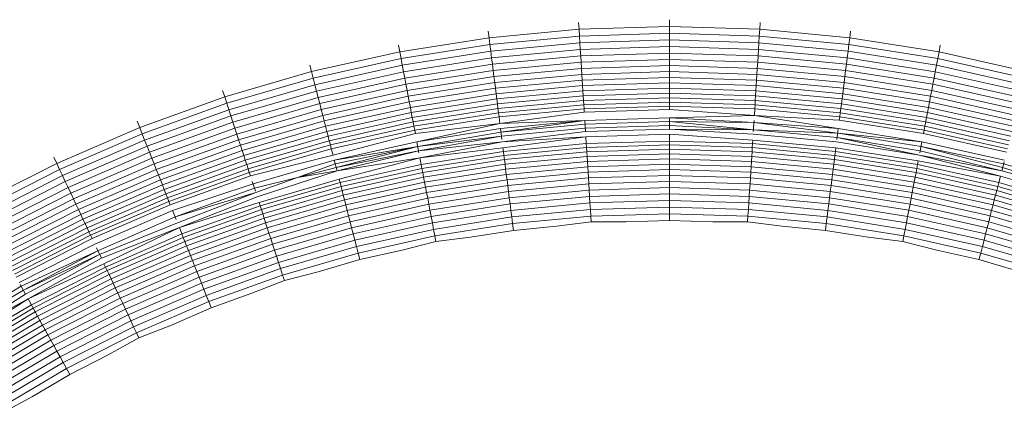
# Model space of a CAD drawing. Units: inches. Extents: x 64 to 1167, y 117 to 939.
# Tile 50 of 56: x 1130.0344 to 1130.3689, y 501.3001 to 501.4339. Entities that reach past the tile are written whole.
import ezdxf

# ---------------------------------------------------------------- set-up
doc = ezdxf.new("R2010")
doc.units = ezdxf.units.IN
doc.header["$MEASUREMENT"] = 0
doc.layers.add('A-FLOR-FIXT', color=8, linetype='Continuous', lineweight=18)

msp = doc.modelspace()

# ---------------------------------------------------------------- linework, layer by layer
at = {"layer": 'A-FLOR-FIXT'}
for p, q in [((1130.25515, 501.4316), (1130.25515, 501.43391)), ((1130.19388, 501.42774), (1130.19359, 501.43003)), ((1130.22445, 501.43064), (1130.19388, 501.42774)), ((1130.22431, 501.43294), (1130.22445, 501.43064)), ((1130.25515, 501.4316), (1130.22445, 501.43064)), ((1130.22445, 501.43064), (1130.2246, 501.42834)), ((1130.25515, 501.4293), (1130.25515, 501.4316)), ((1130.28585, 501.43064), (1130.25515, 501.4316)), ((1130.2857, 501.42834), (1130.28585, 501.43064)), ((1130.28585, 501.43064), (1130.28599, 501.43294)), ((1130.31643, 501.42774), (1130.28585, 501.43064)), ((1130.31643, 501.42774), (1130.31671, 501.43003)), ((1130.19388, 501.42774), (1130.16354, 501.42294)), ((1130.19416, 501.42546), (1130.19388, 501.42774)), ((1130.2246, 501.42834), (1130.19416, 501.42546)), ((1130.25515, 501.4293), (1130.2246, 501.42834)), ((1130.2246, 501.42834), (1130.22474, 501.42607)), ((1130.25515, 501.42702), (1130.22474, 501.42607)), ((1130.25515, 501.42702), (1130.25515, 501.4293)), ((1130.2857, 501.42834), (1130.25515, 501.4293)), ((1130.25515, 501.42477), (1130.25515, 501.42702)), ((1130.28556, 501.42607), (1130.25515, 501.42702)), ((1130.28556, 501.42607), (1130.2857, 501.42834)), ((1130.31614, 501.42546), (1130.2857, 501.42834)), ((1130.31614, 501.42546), (1130.31643, 501.42774)), ((1130.34676, 501.42294), (1130.31643, 501.42774)), ((1130.16311, 501.42521), (1130.16354, 501.42294)), ((1130.19416, 501.42546), (1130.16397, 501.42068)), ((1130.19445, 501.4232), (1130.19416, 501.42546)), ((1130.22474, 501.42607), (1130.19445, 501.4232)), ((1130.22488, 501.42382), (1130.19473, 501.42097)), ((1130.22474, 501.42607), (1130.22488, 501.42382)), ((1130.25515, 501.42477), (1130.22488, 501.42382)), ((1130.22488, 501.42382), (1130.22502, 501.42162)), ((1130.25515, 501.42256), (1130.25515, 501.42477)), ((1130.28542, 501.42382), (1130.25515, 501.42477)), ((1130.28528, 501.42162), (1130.28542, 501.42382)), ((1130.28542, 501.42382), (1130.28556, 501.42607)), ((1130.31557, 501.42097), (1130.28542, 501.42382)), ((1130.31585, 501.4232), (1130.28556, 501.42607)), ((1130.31585, 501.4232), (1130.31614, 501.42546)), ((1130.34633, 501.42068), (1130.31614, 501.42546)), ((1130.34719, 501.42521), (1130.34676, 501.42294)), ((1130.16354, 501.42294), (1130.13357, 501.41624)), ((1130.16397, 501.42068), (1130.13414, 501.41401)), ((1130.16354, 501.42294), (1130.16397, 501.42068)), ((1130.16397, 501.42068), (1130.1644, 501.41844)), ((1130.19445, 501.4232), (1130.1644, 501.41844)), ((1130.19473, 501.42097), (1130.16482, 501.41623)), ((1130.19473, 501.42097), (1130.19445, 501.4232)), ((1130.19501, 501.41878), (1130.19473, 501.42097)), ((1130.22502, 501.42162), (1130.19501, 501.41878)), ((1130.25515, 501.42256), (1130.22502, 501.42162)), ((1130.22502, 501.42162), (1130.22516, 501.41946)), ((1130.25515, 501.4204), (1130.22516, 501.41946)), ((1130.25515, 501.4204), (1130.25515, 501.42256)), ((1130.28528, 501.42162), (1130.25515, 501.42256)), ((1130.25515, 501.4183), (1130.25515, 501.4204)), ((1130.28515, 501.41946), (1130.25515, 501.4204)), ((1130.28515, 501.41946), (1130.28528, 501.42162)), ((1130.31529, 501.41878), (1130.28528, 501.42162)), ((1130.31529, 501.41878), (1130.31557, 501.42097)), ((1130.31557, 501.42097), (1130.31585, 501.4232)), ((1130.34548, 501.41623), (1130.31557, 501.42097)), ((1130.3459, 501.41844), (1130.31585, 501.4232)), ((1130.34633, 501.42068), (1130.3459, 501.41844)), ((1130.34676, 501.42294), (1130.34633, 501.42068)), ((1130.37616, 501.41401), (1130.34633, 501.42068)), ((1130.37673, 501.41624), (1130.34676, 501.42294)), ((1130.13357, 501.41624), (1130.13299, 501.41848)), ((1130.1644, 501.41844), (1130.13471, 501.41181)), ((1130.1644, 501.41844), (1130.16482, 501.41623)), ((1130.19501, 501.41878), (1130.16524, 501.41406)), ((1130.19528, 501.41664), (1130.16564, 501.41194)), ((1130.19528, 501.41664), (1130.19501, 501.41878)), ((1130.22516, 501.41946), (1130.19528, 501.41664)), ((1130.19554, 501.41455), (1130.19528, 501.41664)), ((1130.22529, 501.41736), (1130.19554, 501.41455)), ((1130.22516, 501.41946), (1130.22529, 501.41736)), ((1130.25515, 501.4183), (1130.22529, 501.41736)), ((1130.22529, 501.41736), (1130.22542, 501.41533)), ((1130.25515, 501.41626), (1130.25515, 501.4183)), ((1130.28501, 501.41736), (1130.25515, 501.4183)), ((1130.28489, 501.41533), (1130.28501, 501.41736)), ((1130.28501, 501.41736), (1130.28515, 501.41946)), ((1130.31476, 501.41455), (1130.28501, 501.41736)), ((1130.31502, 501.41664), (1130.28515, 501.41946)), ((1130.31476, 501.41455), (1130.31502, 501.41664)), ((1130.31502, 501.41664), (1130.31529, 501.41878)), ((1130.34466, 501.41194), (1130.31502, 501.41664)), ((1130.34507, 501.41406), (1130.31529, 501.41878)), ((1130.3459, 501.41844), (1130.34548, 501.41623)), ((1130.3756, 501.41181), (1130.3459, 501.41844)), ((1130.13357, 501.41624), (1130.10408, 501.40767)), ((1130.13414, 501.41401), (1130.10479, 501.40549)), ((1130.13414, 501.41401), (1130.13357, 501.41624)), ((1130.13471, 501.41181), (1130.13414, 501.41401)), ((1130.16482, 501.41623), (1130.13527, 501.40963)), ((1130.16524, 501.41406), (1130.13582, 501.40749)), ((1130.16482, 501.41623), (1130.16524, 501.41406)), ((1130.16524, 501.41406), (1130.16564, 501.41194)), ((1130.19554, 501.41455), (1130.16603, 501.40987)), ((1130.1958, 501.41253), (1130.19554, 501.41455)), ((1130.22542, 501.41533), (1130.1958, 501.41253)), ((1130.22554, 501.41337), (1130.19604, 501.41058)), ((1130.25515, 501.41626), (1130.22542, 501.41533)), ((1130.22542, 501.41533), (1130.22554, 501.41337)), ((1130.25515, 501.4143), (1130.22554, 501.41337)), ((1130.22554, 501.41337), (1130.22566, 501.4115)), ((1130.25515, 501.4143), (1130.25515, 501.41626)), ((1130.28489, 501.41533), (1130.25515, 501.41626)), ((1130.25515, 501.41242), (1130.25515, 501.4143)), ((1130.28476, 501.41337), (1130.25515, 501.4143)), ((1130.28464, 501.4115), (1130.28476, 501.41337)), ((1130.28476, 501.41337), (1130.28489, 501.41533)), ((1130.31426, 501.41058), (1130.28476, 501.41337)), ((1130.3145, 501.41253), (1130.28489, 501.41533)), ((1130.3145, 501.41253), (1130.31476, 501.41455)), ((1130.34427, 501.40987), (1130.31476, 501.41455)), ((1130.34507, 501.41406), (1130.34466, 501.41194)), ((1130.34548, 501.41623), (1130.34507, 501.41406)), ((1130.37449, 501.40749), (1130.34507, 501.41406)), ((1130.37504, 501.40963), (1130.34548, 501.41623)), ((1130.13471, 501.41181), (1130.10549, 501.40332)), ((1130.13527, 501.40963), (1130.13471, 501.41181)), ((1130.16564, 501.41194), (1130.13635, 501.40539)), ((1130.16564, 501.41194), (1130.16603, 501.40987)), ((1130.1958, 501.41253), (1130.16642, 501.40787)), ((1130.19604, 501.41058), (1130.16678, 501.40595)), ((1130.19604, 501.41058), (1130.1958, 501.41253)), ((1130.19628, 501.40872), (1130.19604, 501.41058)), ((1130.22566, 501.4115), (1130.19628, 501.40872)), ((1130.25515, 501.41242), (1130.22566, 501.4115)), ((1130.22566, 501.4115), (1130.22577, 501.40971)), ((1130.25515, 501.41064), (1130.22577, 501.40971)), ((1130.25515, 501.41064), (1130.25515, 501.41242)), ((1130.28464, 501.4115), (1130.25515, 501.41242)), ((1130.25515, 501.40895), (1130.25515, 501.41064)), ((1130.28453, 501.40971), (1130.25515, 501.41064)), ((1130.28453, 501.40971), (1130.28464, 501.4115)), ((1130.31402, 501.40872), (1130.28464, 501.4115)), ((1130.31402, 501.40872), (1130.31426, 501.41058)), ((1130.31426, 501.41058), (1130.3145, 501.41253)), ((1130.34352, 501.40595), (1130.31426, 501.41058)), ((1130.34389, 501.40787), (1130.3145, 501.41253)), ((1130.34466, 501.41194), (1130.34427, 501.40987)), ((1130.37395, 501.40539), (1130.34466, 501.41194)), ((1130.10408, 501.40767), (1130.07518, 501.39727)), ((1130.10408, 501.40767), (1130.10336, 501.40987)), ((1130.10479, 501.40549), (1130.10408, 501.40767)), ((1130.13527, 501.40963), (1130.10618, 501.40118)), ((1130.13582, 501.40749), (1130.10687, 501.39908)), ((1130.13582, 501.40749), (1130.13527, 501.40963)), ((1130.13635, 501.40539), (1130.13582, 501.40749)), ((1130.16603, 501.40987), (1130.13688, 501.40336)), ((1130.16642, 501.40787), (1130.13738, 501.40138)), ((1130.16603, 501.40987), (1130.16642, 501.40787)), ((1130.16642, 501.40787), (1130.16678, 501.40595)), ((1130.19628, 501.40872), (1130.16714, 501.4041)), ((1130.1965, 501.40695), (1130.16747, 501.40235)), ((1130.1965, 501.40695), (1130.19628, 501.40872)), ((1130.22577, 501.40971), (1130.1965, 501.40695)), ((1130.19672, 501.40528), (1130.1965, 501.40695)), ((1130.22588, 501.40803), (1130.19672, 501.40528)), ((1130.22577, 501.40971), (1130.22588, 501.40803)), ((1130.25515, 501.40895), (1130.22588, 501.40803)), ((1130.22588, 501.40803), (1130.22597, 501.40646)), ((1130.25515, 501.40737), (1130.22597, 501.40646)), ((1130.25515, 501.40737), (1130.25515, 501.40895)), ((1130.28443, 501.40803), (1130.25515, 501.40895)), ((1130.25515, 501.40591), (1130.25515, 501.40737)), ((1130.28433, 501.40646), (1130.25515, 501.40737)), ((1130.28433, 501.40646), (1130.28443, 501.40803)), ((1130.28443, 501.40803), (1130.28453, 501.40971)), ((1130.31359, 501.40528), (1130.28443, 501.40803)), ((1130.3138, 501.40695), (1130.28453, 501.40971)), ((1130.31359, 501.40528), (1130.3138, 501.40695)), ((1130.3138, 501.40695), (1130.31402, 501.40872)), ((1130.34283, 501.40235), (1130.3138, 501.40695)), ((1130.34317, 501.4041), (1130.31402, 501.40872)), ((1130.34389, 501.40787), (1130.34352, 501.40595)), ((1130.34427, 501.40987), (1130.34389, 501.40787)), ((1130.37292, 501.40138), (1130.34389, 501.40787)), ((1130.37343, 501.40336), (1130.34427, 501.40987)), ((1130.10479, 501.40549), (1130.07602, 501.39513)), ((1130.10549, 501.40332), (1130.07686, 501.39301)), ((1130.10549, 501.40332), (1130.10479, 501.40549)), ((1130.10618, 501.40118), (1130.10549, 501.40332)), ((1130.13635, 501.40539), (1130.10754, 501.39702)), ((1130.13688, 501.40336), (1130.10819, 501.39502)), ((1130.13688, 501.40336), (1130.13635, 501.40539)), ((1130.13738, 501.40138), (1130.13688, 501.40336)), ((1130.16678, 501.40595), (1130.13787, 501.39948)), ((1130.16714, 501.4041), (1130.13834, 501.39767)), ((1130.16678, 501.40595), (1130.16714, 501.4041)), ((1130.16714, 501.4041), (1130.16747, 501.40235)), ((1130.19672, 501.40528), (1130.16779, 501.40069)), ((1130.19691, 501.40371), (1130.16808, 501.39914)), ((1130.19691, 501.40371), (1130.19672, 501.40528)), ((1130.22597, 501.40646), (1130.19691, 501.40371)), ((1130.1971, 501.40226), (1130.19691, 501.40371)), ((1130.22607, 501.40499), (1130.1971, 501.40226)), ((1130.22615, 501.40365), (1130.19727, 501.40092)), ((1130.22597, 501.40646), (1130.22607, 501.40499)), ((1130.25515, 501.40591), (1130.22607, 501.40499)), ((1130.22607, 501.40499), (1130.22615, 501.40365)), ((1130.25515, 501.40456), (1130.22615, 501.40365)), ((1130.22615, 501.40365), (1130.22623, 501.40244)), ((1130.25515, 501.40334), (1130.22623, 501.40244)), ((1130.25515, 501.40456), (1130.25515, 501.40591)), ((1130.28424, 501.40499), (1130.25515, 501.40591)), ((1130.25515, 501.40334), (1130.25515, 501.40456)), ((1130.28415, 501.40365), (1130.25515, 501.40456)), ((1130.28401, 501.40135), (1130.25515, 501.40334)), ((1130.28401, 501.40135), (1130.28415, 501.40365)), ((1130.28415, 501.40365), (1130.28424, 501.40499)), ((1130.31304, 501.40092), (1130.28415, 501.40365)), ((1130.28424, 501.40499), (1130.28433, 501.40646)), ((1130.31321, 501.40226), (1130.28424, 501.40499)), ((1130.31339, 501.40371), (1130.28433, 501.40646)), ((1130.31321, 501.40226), (1130.31339, 501.40371)), ((1130.31339, 501.40371), (1130.31359, 501.40528)), ((1130.34222, 501.39914), (1130.31339, 501.40371)), ((1130.34252, 501.40069), (1130.31359, 501.40528)), ((1130.34317, 501.4041), (1130.34283, 501.40235)), ((1130.34352, 501.40595), (1130.34317, 501.4041)), ((1130.37196, 501.39767), (1130.34317, 501.4041)), ((1130.37243, 501.39948), (1130.34352, 501.40595)), ((1130.10618, 501.40118), (1130.07769, 501.39092)), ((1130.10687, 501.39908), (1130.10618, 501.40118)), ((1130.13738, 501.40138), (1130.10881, 501.39308)), ((1130.13787, 501.39948), (1130.13738, 501.40138)), ((1130.16747, 501.40235), (1130.13878, 501.39594)), ((1130.16779, 501.40069), (1130.1392, 501.3943)), ((1130.16747, 501.40235), (1130.16779, 501.40069)), ((1130.16779, 501.40069), (1130.16808, 501.39914)), ((1130.1971, 501.40226), (1130.16836, 501.3977)), ((1130.19727, 501.40092), (1130.16861, 501.39638)), ((1130.19727, 501.40092), (1130.1971, 501.40226)), ((1130.19755, 501.39863), (1130.19727, 501.40092)), ((1130.22623, 501.40244), (1130.19755, 501.39863)), ((1130.25515, 501.40049), (1130.22641, 501.39959)), ((1130.28401, 501.40135), (1130.25515, 501.40049)), ((1130.28385, 501.39892), (1130.25515, 501.40049)), ((1130.25515, 501.40049), (1130.25515, 501.39674)), ((1130.31288, 501.39971), (1130.28401, 501.40135)), ((1130.31253, 501.39688), (1130.28401, 501.40135)), ((1130.31288, 501.39971), (1130.31304, 501.40092)), ((1130.31304, 501.40092), (1130.31321, 501.40226)), ((1130.34169, 501.39638), (1130.31304, 501.40092)), ((1130.34195, 501.3977), (1130.31321, 501.40226)), ((1130.34252, 501.40069), (1130.34222, 501.39914)), ((1130.34283, 501.40235), (1130.34252, 501.40069)), ((1130.3711, 501.3943), (1130.34252, 501.40069)), ((1130.37152, 501.39594), (1130.34283, 501.40235)), ((1130.07518, 501.39727), (1130.04699, 501.38507)), ((1130.07518, 501.39727), (1130.07433, 501.39941)), ((1130.07602, 501.39513), (1130.07518, 501.39727)), ((1130.10687, 501.39908), (1130.0785, 501.38887)), ((1130.10754, 501.39702), (1130.0793, 501.38686)), ((1130.10754, 501.39702), (1130.10687, 501.39908)), ((1130.10819, 501.39502), (1130.10754, 501.39702)), ((1130.13787, 501.39948), (1130.10942, 501.39122)), ((1130.13834, 501.39767), (1130.11, 501.38943)), ((1130.13787, 501.39948), (1130.13834, 501.39767)), ((1130.13834, 501.39767), (1130.13878, 501.39594)), ((1130.16808, 501.39914), (1130.13959, 501.39278)), ((1130.16836, 501.3977), (1130.13996, 501.39136)), ((1130.16808, 501.39914), (1130.16836, 501.3977)), ((1130.16836, 501.3977), (1130.16861, 501.39638)), ((1130.19755, 501.39863), (1130.16884, 501.39518)), ((1130.19755, 501.39863), (1130.16937, 501.39238)), ((1130.19778, 501.39688), (1130.16937, 501.39238)), ((1130.22641, 501.39959), (1130.19755, 501.39863)), ((1130.22641, 501.39959), (1130.19778, 501.39688)), ((1130.19778, 501.39688), (1130.19825, 501.39316)), ((1130.22641, 501.39959), (1130.19793, 501.39569)), ((1130.22648, 501.39839), (1130.19793, 501.39569)), ((1130.22657, 501.39704), (1130.1981, 501.39435)), ((1130.22641, 501.39959), (1130.22664, 501.39585)), ((1130.25515, 501.39929), (1130.22648, 501.39839)), ((1130.25515, 501.39794), (1130.22657, 501.39704)), ((1130.25515, 501.39674), (1130.22664, 501.39585)), ((1130.28385, 501.39892), (1130.25515, 501.39929)), ((1130.2837, 501.39652), (1130.25515, 501.39929)), ((1130.2837, 501.39652), (1130.25515, 501.39794)), ((1130.28361, 501.39503), (1130.25515, 501.39674)), ((1130.2837, 501.39652), (1130.25515, 501.39674)), ((1130.2839, 501.39959), (1130.28366, 501.39585)), ((1130.31214, 501.39383), (1130.2837, 501.39652)), ((1130.31233, 501.39532), (1130.2837, 501.39652)), ((1130.31233, 501.39532), (1130.28385, 501.39892)), ((1130.31253, 501.39688), (1130.28385, 501.39892)), ((1130.31253, 501.39688), (1130.31206, 501.39316)), ((1130.34093, 501.39238), (1130.31253, 501.39688)), ((1130.34147, 501.39518), (1130.31288, 501.39971)), ((1130.34195, 501.3977), (1130.34169, 501.39638)), ((1130.34222, 501.39914), (1130.34195, 501.3977)), ((1130.37034, 501.39136), (1130.34195, 501.3977)), ((1130.37071, 501.39278), (1130.34222, 501.39914)), ((1130.07602, 501.39513), (1130.04797, 501.38299)), ((1130.07686, 501.39301), (1130.07602, 501.39513)), ((1130.10819, 501.39502), (1130.08007, 501.3849)), ((1130.10881, 501.39308), (1130.10819, 501.39502)), ((1130.13878, 501.39594), (1130.11055, 501.38774)), ((1130.1392, 501.3943), (1130.11107, 501.38613)), ((1130.13878, 501.39594), (1130.1392, 501.3943)), ((1130.1392, 501.3943), (1130.13959, 501.39278)), ((1130.16861, 501.39638), (1130.14029, 501.39005)), ((1130.16884, 501.39518), (1130.14087, 501.38782)), ((1130.16861, 501.39638), (1130.16884, 501.39518)), ((1130.19793, 501.39569), (1130.16967, 501.39084)), ((1130.1981, 501.39435), (1130.16967, 501.39084)), ((1130.1981, 501.39435), (1130.16995, 501.38936)), ((1130.22664, 501.39585), (1130.19835, 501.39236)), ((1130.22675, 501.39408), (1130.19835, 501.39236)), ((1130.22675, 501.39408), (1130.1986, 501.39033)), ((1130.25515, 501.39498), (1130.22675, 501.39408)), ((1130.2269, 501.39178), (1130.22675, 501.39408)), ((1130.25515, 501.39498), (1130.25515, 501.39267)), ((1130.28348, 501.393), (1130.25515, 501.39498)), ((1130.31195, 501.39236), (1130.28361, 501.39503)), ((1130.34008, 501.3879), (1130.31214, 501.39383)), ((1130.34035, 501.38936), (1130.31214, 501.39383)), ((1130.34093, 501.39238), (1130.31233, 501.39532)), ((1130.34064, 501.39084), (1130.31233, 501.39532)), ((1130.34169, 501.39638), (1130.34147, 501.39518)), ((1130.36971, 501.38887), (1130.34147, 501.39518)), ((1130.37001, 501.39005), (1130.34169, 501.39638)), ((1130.07686, 501.39301), (1130.04894, 501.38093)), ((1130.07769, 501.39092), (1130.0499, 501.37889)), ((1130.07769, 501.39092), (1130.07686, 501.39301)), ((1130.0785, 501.38887), (1130.07769, 501.39092)), ((1130.10881, 501.39308), (1130.08082, 501.38301)), ((1130.10942, 501.39122), (1130.08155, 501.38118)), ((1130.10942, 501.39122), (1130.10881, 501.39308)), ((1130.11, 501.38943), (1130.10942, 501.39122)), ((1130.13959, 501.39278), (1130.11156, 501.38463)), ((1130.13996, 501.39136), (1130.11201, 501.38324)), ((1130.14029, 501.39005), (1130.11243, 501.38196)), ((1130.13959, 501.39278), (1130.13996, 501.39136)), ((1130.13996, 501.39136), (1130.14029, 501.39005)), ((1130.14029, 501.39005), (1130.14087, 501.38782)), ((1130.16937, 501.39238), (1130.14131, 501.38611)), ((1130.16967, 501.39084), (1130.14131, 501.38611)), ((1130.16967, 501.39084), (1130.1416, 501.38495)), ((1130.16967, 501.39084), (1130.14194, 501.38364)), ((1130.16937, 501.39238), (1130.17007, 501.3887)), ((1130.19835, 501.39236), (1130.16995, 501.38936)), ((1130.19835, 501.39236), (1130.1704, 501.38697)), ((1130.1986, 501.39033), (1130.1704, 501.38697)), ((1130.19876, 501.38912), (1130.1986, 501.39033)), ((1130.2269, 501.39178), (1130.19876, 501.38912)), ((1130.22698, 501.39044), (1130.19892, 501.38779)), ((1130.25515, 501.39267), (1130.2269, 501.39178)), ((1130.22698, 501.39044), (1130.2269, 501.39178)), ((1130.25515, 501.39132), (1130.22698, 501.39044)), ((1130.22707, 501.38898), (1130.22698, 501.39044)), ((1130.25515, 501.38986), (1130.22707, 501.38898)), ((1130.25515, 501.39267), (1130.25515, 501.39132)), ((1130.2834, 501.39178), (1130.25515, 501.39267)), ((1130.25515, 501.39132), (1130.25515, 501.38986)), ((1130.28332, 501.39044), (1130.25515, 501.39132)), ((1130.25515, 501.38986), (1130.25515, 501.38828)), ((1130.28323, 501.38898), (1130.25515, 501.38986)), ((1130.28323, 501.38898), (1130.28332, 501.39044)), ((1130.28332, 501.39044), (1130.2834, 501.39178)), ((1130.31138, 501.38779), (1130.28332, 501.39044)), ((1130.2834, 501.39178), (1130.28348, 501.393)), ((1130.31155, 501.38912), (1130.2834, 501.39178)), ((1130.3117, 501.39033), (1130.28348, 501.393)), ((1130.31155, 501.38912), (1130.3117, 501.39033)), ((1130.33969, 501.3859), (1130.3117, 501.39033)), ((1130.34008, 501.3879), (1130.31195, 501.39236)), ((1130.34093, 501.39238), (1130.34023, 501.3887)), ((1130.3687, 501.38495), (1130.34064, 501.39084)), ((1130.36836, 501.38364), (1130.34064, 501.39084)), ((1130.369, 501.38611), (1130.34093, 501.39238)), ((1130.04699, 501.38507), (1130.04601, 501.38716)), ((1130.0785, 501.38887), (1130.05084, 501.37689)), ((1130.0793, 501.38686), (1130.05176, 501.37494)), ((1130.0793, 501.38686), (1130.0785, 501.38887)), ((1130.08007, 501.3849), (1130.0793, 501.38686)), ((1130.11, 501.38943), (1130.08224, 501.37944)), ((1130.11055, 501.38774), (1130.08289, 501.37778)), ((1130.11055, 501.38774), (1130.11, 501.38943)), ((1130.11107, 501.38613), (1130.11055, 501.38774)), ((1130.14087, 501.38782), (1130.11281, 501.3808)), ((1130.16995, 501.38936), (1130.14194, 501.38364)), ((1130.16995, 501.38936), (1130.14224, 501.38248)), ((1130.1704, 501.38697), (1130.14224, 501.38248)), ((1130.1704, 501.38697), (1130.14295, 501.37971)), ((1130.1704, 501.38697), (1130.17084, 501.3847)), ((1130.19876, 501.38912), (1130.17084, 501.3847)), ((1130.19892, 501.38779), (1130.17109, 501.38338)), ((1130.19892, 501.38779), (1130.19876, 501.38912)), ((1130.19911, 501.38633), (1130.19892, 501.38779)), ((1130.22707, 501.38898), (1130.19911, 501.38633)), ((1130.22717, 501.3874), (1130.19931, 501.38477)), ((1130.22717, 501.3874), (1130.22707, 501.38898)), ((1130.25515, 501.38828), (1130.22717, 501.3874)), ((1130.22728, 501.38572), (1130.22717, 501.3874)), ((1130.25515, 501.38659), (1130.22728, 501.38572)), ((1130.25515, 501.38828), (1130.25515, 501.38659)), ((1130.28313, 501.3874), (1130.25515, 501.38828)), ((1130.25515, 501.38659), (1130.25515, 501.38481)), ((1130.28302, 501.38572), (1130.25515, 501.38659)), ((1130.28302, 501.38572), (1130.28313, 501.3874)), ((1130.28313, 501.3874), (1130.28323, 501.38898)), ((1130.311, 501.38477), (1130.28313, 501.3874)), ((1130.31119, 501.38633), (1130.28323, 501.38898)), ((1130.31119, 501.38633), (1130.31138, 501.38779)), ((1130.31138, 501.38779), (1130.31155, 501.38912)), ((1130.33921, 501.38338), (1130.31138, 501.38779)), ((1130.33947, 501.3847), (1130.31155, 501.38912)), ((1130.36763, 501.38077), (1130.34008, 501.3879)), ((1130.36807, 501.38248), (1130.34008, 501.3879)), ((1130.36807, 501.38248), (1130.34035, 501.38936)), ((1130.04699, 501.38507), (1130.01963, 501.37113)), ((1130.04797, 501.38299), (1130.04699, 501.38507)), ((1130.08007, 501.3849), (1130.05265, 501.37304)), ((1130.08082, 501.38301), (1130.08007, 501.3849)), ((1130.11107, 501.38613), (1130.08351, 501.37621)), ((1130.11156, 501.38463), (1130.0841, 501.37474)), ((1130.11201, 501.38324), (1130.08464, 501.37338)), ((1130.11156, 501.38463), (1130.11107, 501.38613)), ((1130.11201, 501.38324), (1130.11156, 501.38463)), ((1130.11243, 501.38196), (1130.11201, 501.38324)), ((1130.14131, 501.38611), (1130.11369, 501.37808)), ((1130.1416, 501.38495), (1130.12881, 501.3803)), ((1130.14194, 501.38364), (1130.12881, 501.3803)), ((1130.14131, 501.38611), (1130.14224, 501.38248)), ((1130.17084, 501.3847), (1130.14325, 501.37853)), ((1130.17109, 501.38338), (1130.14359, 501.37723)), ((1130.17084, 501.3847), (1130.17109, 501.38338)), ((1130.17109, 501.38338), (1130.17136, 501.38194)), ((1130.19911, 501.38633), (1130.17136, 501.38194)), ((1130.19931, 501.38477), (1130.17166, 501.38039)), ((1130.19931, 501.38477), (1130.19911, 501.38633)), ((1130.19952, 501.38309), (1130.19931, 501.38477)), ((1130.22728, 501.38572), (1130.19952, 501.38309)), ((1130.22739, 501.38394), (1130.19974, 501.38132)), ((1130.22739, 501.38394), (1130.22728, 501.38572)), ((1130.25515, 501.38481), (1130.22739, 501.38394)), ((1130.22751, 501.38206), (1130.22739, 501.38394)), ((1130.25515, 501.38481), (1130.25515, 501.38293)), ((1130.28291, 501.38394), (1130.25515, 501.38481)), ((1130.28279, 501.38206), (1130.28291, 501.38394)), ((1130.28291, 501.38394), (1130.28302, 501.38572)), ((1130.31056, 501.38132), (1130.28291, 501.38394)), ((1130.31078, 501.38309), (1130.28302, 501.38572)), ((1130.31078, 501.38309), (1130.311, 501.38477)), ((1130.311, 501.38477), (1130.31119, 501.38633)), ((1130.33864, 501.38039), (1130.311, 501.38477)), ((1130.33894, 501.38194), (1130.31119, 501.38633)), ((1130.33894, 501.38194), (1130.33921, 501.38338)), ((1130.33921, 501.38338), (1130.33947, 501.3847)), ((1130.36672, 501.37723), (1130.33921, 501.38338)), ((1130.33947, 501.3847), (1130.33969, 501.3859)), ((1130.36705, 501.37853), (1130.33947, 501.3847)), ((1130.36763, 501.38077), (1130.33969, 501.3859)), ((1130.36886, 501.38558), (1130.36807, 501.38248)), ((1130.39566, 501.37516), (1130.36836, 501.38364)), ((1130.39624, 501.37695), (1130.3687, 501.38495)), ((1130.04797, 501.38299), (1130.02073, 501.36911)), ((1130.04894, 501.38093), (1130.02183, 501.36712)), ((1130.04894, 501.38093), (1130.04797, 501.38299)), ((1130.0499, 501.37889), (1130.04894, 501.38093)), ((1130.08082, 501.38301), (1130.05352, 501.37119)), ((1130.08155, 501.38118), (1130.05436, 501.36942)), ((1130.08155, 501.38118), (1130.08082, 501.38301)), ((1130.08224, 501.37944), (1130.08155, 501.38118)), ((1130.11243, 501.38196), (1130.08513, 501.37213)), ((1130.11281, 501.3808), (1130.08558, 501.371)), ((1130.11281, 501.3808), (1130.11243, 501.38196)), ((1130.12881, 501.3803), (1130.11417, 501.37659)), ((1130.12881, 501.3803), (1130.11464, 501.37516)), ((1130.14224, 501.38248), (1130.1151, 501.37375)), ((1130.14224, 501.38248), (1130.12881, 501.3803)), ((1130.17136, 501.38194), (1130.14395, 501.37581)), ((1130.17166, 501.38039), (1130.14434, 501.37428)), ((1130.17166, 501.38039), (1130.17136, 501.38194)), ((1130.17198, 501.37873), (1130.17166, 501.38039)), ((1130.19952, 501.38309), (1130.17198, 501.37873)), ((1130.19974, 501.38132), (1130.17231, 501.37698)), ((1130.19974, 501.38132), (1130.19952, 501.38309)), ((1130.19998, 501.37946), (1130.19974, 501.38132)), ((1130.22751, 501.38206), (1130.19998, 501.37946)), ((1130.22763, 501.3801), (1130.20022, 501.37751)), ((1130.25515, 501.38293), (1130.22751, 501.38206)), ((1130.22763, 501.3801), (1130.22751, 501.38206)), ((1130.25515, 501.38097), (1130.22763, 501.3801)), ((1130.22776, 501.37807), (1130.22763, 501.3801)), ((1130.25515, 501.38293), (1130.25515, 501.38097)), ((1130.28279, 501.38206), (1130.25515, 501.38293)), ((1130.25515, 501.38097), (1130.25515, 501.37893)), ((1130.28267, 501.3801), (1130.25515, 501.38097)), ((1130.28254, 501.37807), (1130.28267, 501.3801)), ((1130.28267, 501.3801), (1130.28279, 501.38206)), ((1130.31008, 501.37751), (1130.28267, 501.3801)), ((1130.31033, 501.37946), (1130.28279, 501.38206)), ((1130.31033, 501.37946), (1130.31056, 501.38132)), ((1130.31056, 501.38132), (1130.31078, 501.38309)), ((1130.33799, 501.37698), (1130.31056, 501.38132)), ((1130.33833, 501.37873), (1130.31078, 501.38309)), ((1130.33833, 501.37873), (1130.33864, 501.38039)), ((1130.33864, 501.38039), (1130.33894, 501.38194)), ((1130.36596, 501.37428), (1130.33864, 501.38039)), ((1130.36635, 501.37581), (1130.33894, 501.38194)), ((1130.36705, 501.37853), (1130.36763, 501.38077)), ((1130.39491, 501.37284), (1130.36763, 501.38077)), ((1130.39566, 501.37516), (1130.36807, 501.38248)), ((1130.0499, 501.37889), (1130.02291, 501.36515)), ((1130.05084, 501.37689), (1130.02398, 501.36321)), ((1130.05084, 501.37689), (1130.0499, 501.37889)), ((1130.05176, 501.37494), (1130.05084, 501.37689)), ((1130.08224, 501.37944), (1130.05516, 501.36772)), ((1130.08289, 501.37778), (1130.05592, 501.3661)), ((1130.08289, 501.37778), (1130.08224, 501.37944)), ((1130.08351, 501.37621), (1130.08289, 501.37778)), ((1130.11369, 501.37808), (1130.08633, 501.3691)), ((1130.11417, 501.37659), (1130.08721, 501.36688)), ((1130.11344, 501.37886), (1130.11448, 501.37566)), ((1130.14295, 501.37971), (1130.11573, 501.37181)), ((1130.14325, 501.37853), (1130.11611, 501.37065)), ((1130.14359, 501.37723), (1130.11652, 501.36937)), ((1130.14325, 501.37853), (1130.14295, 501.37971)), ((1130.14359, 501.37723), (1130.14325, 501.37853)), ((1130.14395, 501.37581), (1130.14359, 501.37723)), ((1130.17198, 501.37873), (1130.14476, 501.37265)), ((1130.17231, 501.37698), (1130.14521, 501.37092)), ((1130.17231, 501.37698), (1130.17198, 501.37873)), ((1130.17266, 501.37513), (1130.17231, 501.37698)), ((1130.19998, 501.37946), (1130.17266, 501.37513)), ((1130.20022, 501.37751), (1130.17303, 501.37321)), ((1130.20022, 501.37751), (1130.19998, 501.37946)), ((1130.20048, 501.37549), (1130.20022, 501.37751)), ((1130.22776, 501.37807), (1130.20048, 501.37549)), ((1130.25515, 501.37893), (1130.22776, 501.37807)), ((1130.22789, 501.37597), (1130.22776, 501.37807)), ((1130.25515, 501.37683), (1130.22789, 501.37597)), ((1130.25515, 501.37893), (1130.25515, 501.37683)), ((1130.28254, 501.37807), (1130.25515, 501.37893)), ((1130.25515, 501.37683), (1130.25515, 501.37467)), ((1130.28241, 501.37597), (1130.25515, 501.37683)), ((1130.28241, 501.37597), (1130.28254, 501.37807)), ((1130.30982, 501.37549), (1130.28254, 501.37807)), ((1130.30982, 501.37549), (1130.31008, 501.37751)), ((1130.31008, 501.37751), (1130.31033, 501.37946)), ((1130.33727, 501.37321), (1130.31008, 501.37751)), ((1130.33764, 501.37513), (1130.31033, 501.37946)), ((1130.33764, 501.37513), (1130.33799, 501.37698)), ((1130.33799, 501.37698), (1130.33833, 501.37873)), ((1130.3651, 501.37092), (1130.33799, 501.37698)), ((1130.36554, 501.37265), (1130.33833, 501.37873)), ((1130.36635, 501.37581), (1130.36672, 501.37723)), ((1130.36672, 501.37723), (1130.36705, 501.37853)), ((1130.39378, 501.36937), (1130.36672, 501.37723)), ((1130.3942, 501.37065), (1130.36705, 501.37853)), ((1130.05176, 501.37494), (1130.02502, 501.36131)), ((1130.05265, 501.37304), (1130.05176, 501.37494)), ((1130.08351, 501.37621), (1130.05663, 501.36458)), ((1130.0841, 501.37474), (1130.05731, 501.36315)), ((1130.08464, 501.37338), (1130.05793, 501.36182)), ((1130.0841, 501.37474), (1130.08351, 501.37621)), ((1130.08464, 501.37338), (1130.0841, 501.37474)), ((1130.08513, 501.37213), (1130.08464, 501.37338)), ((1130.11464, 501.37516), (1130.08721, 501.36688)), ((1130.11464, 501.37516), (1130.08801, 501.36486)), ((1130.1151, 501.37375), (1130.08866, 501.36322)), ((1130.14395, 501.37581), (1130.11697, 501.36797)), ((1130.14434, 501.37428), (1130.11746, 501.36647)), ((1130.14434, 501.37428), (1130.14395, 501.37581)), ((1130.14434, 501.37428), (1130.14476, 501.37265)), ((1130.17266, 501.37513), (1130.14567, 501.3691)), ((1130.17303, 501.37321), (1130.14616, 501.3672)), ((1130.17303, 501.37321), (1130.17266, 501.37513)), ((1130.17341, 501.37121), (1130.17303, 501.37321)), ((1130.20048, 501.37549), (1130.17341, 501.37121)), ((1130.20074, 501.37341), (1130.1738, 501.36914)), ((1130.20074, 501.37341), (1130.20048, 501.37549)), ((1130.22789, 501.37597), (1130.20074, 501.37341)), ((1130.20101, 501.37126), (1130.20074, 501.37341)), ((1130.22803, 501.37382), (1130.20101, 501.37126)), ((1130.22803, 501.37382), (1130.22789, 501.37597)), ((1130.25515, 501.37467), (1130.22803, 501.37382)), ((1130.22817, 501.37161), (1130.22803, 501.37382)), ((1130.25515, 501.37467), (1130.25515, 501.37246)), ((1130.28227, 501.37382), (1130.25515, 501.37467)), ((1130.28214, 501.37161), (1130.28227, 501.37382)), ((1130.28227, 501.37382), (1130.28241, 501.37597)), ((1130.30929, 501.37126), (1130.28227, 501.37382)), ((1130.30956, 501.37341), (1130.28241, 501.37597)), ((1130.30929, 501.37126), (1130.30956, 501.37341)), ((1130.30956, 501.37341), (1130.30982, 501.37549)), ((1130.3365, 501.36914), (1130.30956, 501.37341)), ((1130.33689, 501.37121), (1130.30982, 501.37549)), ((1130.33689, 501.37121), (1130.33727, 501.37321)), ((1130.33727, 501.37321), (1130.33764, 501.37513)), ((1130.36414, 501.3672), (1130.33727, 501.37321)), ((1130.36463, 501.3691), (1130.33764, 501.37513)), ((1130.36554, 501.37265), (1130.36596, 501.37428)), ((1130.36596, 501.37428), (1130.36635, 501.37581)), ((1130.39284, 501.36647), (1130.36596, 501.37428)), ((1130.39333, 501.36797), (1130.36635, 501.37581)), ((1130.05265, 501.37304), (1130.02603, 501.35947)), ((1130.05352, 501.37119), (1130.02701, 501.35769)), ((1130.05352, 501.37119), (1130.05265, 501.37304)), ((1130.05436, 501.36942), (1130.05352, 501.37119)), ((1130.08513, 501.37213), (1130.0585, 501.36061)), ((1130.08558, 501.371), (1130.05902, 501.3595)), ((1130.08558, 501.371), (1130.08513, 501.37213)), ((1130.11573, 501.37181), (1130.08866, 501.36322)), ((1130.11611, 501.37065), (1130.08951, 501.36107)), ((1130.11611, 501.37065), (1130.11573, 501.37181)), ((1130.11652, 501.36937), (1130.11611, 501.37065)), ((1130.14476, 501.37265), (1130.11798, 501.36487)), ((1130.14521, 501.37092), (1130.11853, 501.36317)), ((1130.14476, 501.37265), (1130.14521, 501.37092)), ((1130.14521, 501.37092), (1130.14567, 501.3691)), ((1130.17341, 501.37121), (1130.14667, 501.36523)), ((1130.1738, 501.36914), (1130.17341, 501.37121)), ((1130.20101, 501.37126), (1130.17421, 501.36702)), ((1130.20129, 501.36907), (1130.20101, 501.37126)), ((1130.22817, 501.37161), (1130.20129, 501.36907)), ((1130.25515, 501.37246), (1130.22817, 501.37161)), ((1130.22831, 501.36937), (1130.22817, 501.37161)), ((1130.25515, 501.37021), (1130.22831, 501.36937)), ((1130.25515, 501.37246), (1130.25515, 501.37021)), ((1130.28214, 501.37161), (1130.25515, 501.37246)), ((1130.25515, 501.37021), (1130.25515, 501.36793)), ((1130.28199, 501.36937), (1130.25515, 501.37021)), ((1130.28199, 501.36937), (1130.28214, 501.37161)), ((1130.30901, 501.36907), (1130.28214, 501.37161)), ((1130.30901, 501.36907), (1130.30929, 501.37126)), ((1130.33609, 501.36702), (1130.30929, 501.37126)), ((1130.3365, 501.36914), (1130.33689, 501.37121)), ((1130.36364, 501.36523), (1130.33689, 501.37121)), ((1130.36463, 501.3691), (1130.3651, 501.37092)), ((1130.3651, 501.37092), (1130.36554, 501.37265)), ((1130.39177, 501.36317), (1130.3651, 501.37092)), ((1130.39232, 501.36487), (1130.36554, 501.37265)), ((1130.05436, 501.36942), (1130.02796, 501.35597)), ((1130.05516, 501.36772), (1130.02886, 501.35432)), ((1130.05516, 501.36772), (1130.05436, 501.36942)), ((1130.05592, 501.3661), (1130.05516, 501.36772)), ((1130.08633, 501.3691), (1130.05989, 501.35766)), ((1130.08721, 501.36688), (1130.061, 501.35529)), ((1130.08633, 501.3691), (1130.08757, 501.36597)), ((1130.11652, 501.36937), (1130.09, 501.35982)), ((1130.11697, 501.36797), (1130.09054, 501.35846)), ((1130.11746, 501.36647), (1130.09113, 501.35699)), ((1130.11697, 501.36797), (1130.11652, 501.36937)), ((1130.11746, 501.36647), (1130.11697, 501.36797)), ((1130.11798, 501.36487), (1130.11746, 501.36647)), ((1130.14567, 501.3691), (1130.11911, 501.36138)), ((1130.14616, 501.3672), (1130.11972, 501.35952)), ((1130.14567, 501.3691), (1130.14616, 501.3672)), ((1130.14616, 501.3672), (1130.14667, 501.36523)), ((1130.1738, 501.36914), (1130.14719, 501.36319)), ((1130.17421, 501.36702), (1130.14773, 501.3611)), ((1130.17421, 501.36702), (1130.1738, 501.36914)), ((1130.17462, 501.36485), (1130.17421, 501.36702)), ((1130.20129, 501.36907), (1130.17462, 501.36485)), ((1130.20157, 501.36684), (1130.17505, 501.36264)), ((1130.20157, 501.36684), (1130.20129, 501.36907)), ((1130.22831, 501.36937), (1130.20157, 501.36684)), ((1130.20186, 501.36458), (1130.20157, 501.36684)), ((1130.22845, 501.36709), (1130.20186, 501.36458)), ((1130.22845, 501.36709), (1130.22831, 501.36937)), ((1130.25515, 501.36793), (1130.22845, 501.36709)), ((1130.22857, 501.36517), (1130.22845, 501.36709)), ((1130.25515, 501.36793), (1130.25515, 501.36563)), ((1130.28185, 501.36709), (1130.25515, 501.36793)), ((1130.28173, 501.36517), (1130.28185, 501.36709)), ((1130.28185, 501.36709), (1130.28199, 501.36937)), ((1130.30845, 501.36458), (1130.28185, 501.36709)), ((1130.30873, 501.36684), (1130.28199, 501.36937)), ((1130.30845, 501.36458), (1130.30873, 501.36684)), ((1130.30873, 501.36684), (1130.30901, 501.36907)), ((1130.33526, 501.36264), (1130.30873, 501.36684)), ((1130.33568, 501.36485), (1130.30901, 501.36907)), ((1130.33568, 501.36485), (1130.33609, 501.36702)), ((1130.33609, 501.36702), (1130.3365, 501.36914)), ((1130.36258, 501.3611), (1130.33609, 501.36702)), ((1130.36311, 501.36319), (1130.3365, 501.36914)), ((1130.36364, 501.36523), (1130.36414, 501.3672)), ((1130.36414, 501.3672), (1130.36463, 501.3691)), ((1130.39058, 501.35952), (1130.36414, 501.3672)), ((1130.39119, 501.36138), (1130.36463, 501.3691)), ((1130.05592, 501.3661), (1130.02972, 501.35276)), ((1130.05663, 501.36458), (1130.03054, 501.35128)), ((1130.05731, 501.36315), (1130.0313, 501.3499)), ((1130.05663, 501.36458), (1130.05592, 501.3661)), ((1130.05731, 501.36315), (1130.05663, 501.36458)), ((1130.05793, 501.36182), (1130.05731, 501.36315)), ((1130.08801, 501.36486), (1130.06155, 501.35414)), ((1130.08866, 501.36322), (1130.06218, 501.35279)), ((1130.08866, 501.36322), (1130.06305, 501.35095)), ((1130.08951, 501.36107), (1130.08866, 501.36322)), ((1130.11798, 501.36487), (1130.09175, 501.35542)), ((1130.11853, 501.36317), (1130.0924, 501.35376)), ((1130.11853, 501.36317), (1130.11798, 501.36487)), ((1130.11911, 501.36138), (1130.11853, 501.36317)), ((1130.14667, 501.36523), (1130.12035, 501.35758)), ((1130.14719, 501.36319), (1130.121, 501.35558)), ((1130.14667, 501.36523), (1130.14719, 501.36319)), ((1130.14719, 501.36319), (1130.14773, 501.3611)), ((1130.17462, 501.36485), (1130.14828, 501.35896)), ((1130.17505, 501.36264), (1130.17462, 501.36485)), ((1130.20186, 501.36458), (1130.17547, 501.3604)), ((1130.20214, 501.3623), (1130.20186, 501.36458)), ((1130.21679, 501.36368), (1130.20214, 501.3623)), ((1130.22857, 501.36517), (1130.21679, 501.36368)), ((1130.24044, 501.36517), (1130.22857, 501.36517)), ((1130.25515, 501.36563), (1130.24044, 501.36517)), ((1130.26986, 501.36517), (1130.25515, 501.36563)), ((1130.28173, 501.36517), (1130.26986, 501.36517)), ((1130.29351, 501.36368), (1130.28173, 501.36517)), ((1130.30816, 501.3623), (1130.29351, 501.36368)), ((1130.30816, 501.3623), (1130.30845, 501.36458)), ((1130.33483, 501.3604), (1130.30845, 501.36458)), ((1130.33526, 501.36264), (1130.33568, 501.36485)), ((1130.36203, 501.35896), (1130.33568, 501.36485)), ((1130.36258, 501.3611), (1130.36311, 501.36319)), ((1130.36311, 501.36319), (1130.36364, 501.36523)), ((1130.3893, 501.35558), (1130.36311, 501.36319)), ((1130.38995, 501.35758), (1130.36364, 501.36523)), ((1130.05793, 501.36182), (1130.032, 501.34861)), ((1130.0585, 501.36061), (1130.03265, 501.34744)), ((1130.0585, 501.36061), (1130.05793, 501.36182)), ((1130.05902, 501.3595), (1130.0585, 501.36061)), ((1130.08951, 501.36107), (1130.06357, 501.34984)), ((1130.09, 501.35982), (1130.06414, 501.34863)), ((1130.09, 501.35982), (1130.08951, 501.36107)), ((1130.09054, 501.35846), (1130.09, 501.35982)), ((1130.11911, 501.36138), (1130.09309, 501.35202)), ((1130.11972, 501.35952), (1130.11911, 501.36138)), ((1130.14773, 501.3611), (1130.12167, 501.35353)), ((1130.14773, 501.3611), (1130.14828, 501.35896)), ((1130.17505, 501.36264), (1130.14884, 501.35678)), ((1130.17547, 501.3604), (1130.1494, 501.35457)), ((1130.17547, 501.3604), (1130.17505, 501.36264)), ((1130.17583, 501.35851), (1130.17547, 501.3604)), ((1130.18761, 501.36), (1130.17583, 501.35851)), ((1130.20214, 501.3623), (1130.18761, 501.36)), ((1130.32269, 501.36), (1130.30816, 501.3623)), ((1130.33447, 501.35851), (1130.32269, 501.36)), ((1130.33447, 501.35851), (1130.33483, 501.3604)), ((1130.33483, 501.3604), (1130.33526, 501.36264)), ((1130.3609, 501.35457), (1130.33483, 501.3604)), ((1130.36147, 501.35678), (1130.33526, 501.36264)), ((1130.36203, 501.35896), (1130.36258, 501.3611)), ((1130.38863, 501.35353), (1130.36258, 501.3611)), ((1130.05902, 501.3595), (1130.03324, 501.34637)), ((1130.05989, 501.35766), (1130.03422, 501.34458)), ((1130.09054, 501.35846), (1130.06476, 501.3473)), ((1130.09113, 501.35699), (1130.06544, 501.34587)), ((1130.09113, 501.35699), (1130.09054, 501.35846)), ((1130.09175, 501.35542), (1130.09113, 501.35699)), ((1130.11972, 501.35952), (1130.09382, 501.35019)), ((1130.12035, 501.35758), (1130.09457, 501.3483)), ((1130.12035, 501.35758), (1130.11972, 501.35952)), ((1130.121, 501.35558), (1130.12035, 501.35758)), ((1130.14828, 501.35896), (1130.12235, 501.35142)), ((1130.14884, 501.35678), (1130.12305, 501.34929)), ((1130.14828, 501.35896), (1130.14884, 501.35678)), ((1130.14884, 501.35678), (1130.1494, 501.35457)), ((1130.17583, 501.35851), (1130.16433, 501.35555)), ((1130.34597, 501.35555), (1130.33447, 501.35851)), ((1130.3609, 501.35457), (1130.36147, 501.35678)), ((1130.36147, 501.35678), (1130.36203, 501.35896)), ((1130.38726, 501.34929), (1130.36147, 501.35678)), ((1130.38795, 501.35142), (1130.36203, 501.35896)), ((1130.061, 501.35529), (1130.03494, 501.34328)), ((1130.061, 501.35529), (1130.03566, 501.34196)), ((1130.06155, 501.35414), (1130.03566, 501.34196)), ((1130.06155, 501.35414), (1130.03642, 501.34058)), ((1130.06052, 501.35631), (1130.06218, 501.35279)), ((1130.09175, 501.35542), (1130.06615, 501.34435)), ((1130.0924, 501.35376), (1130.06691, 501.34273)), ((1130.0924, 501.35376), (1130.09175, 501.35542)), ((1130.09309, 501.35202), (1130.0924, 501.35376)), ((1130.121, 501.35558), (1130.09534, 501.34634)), ((1130.12167, 501.35353), (1130.09614, 501.34433)), ((1130.12167, 501.35353), (1130.121, 501.35558)), ((1130.12235, 501.35142), (1130.12167, 501.35353)), ((1130.1494, 501.35457), (1130.12375, 501.34712)), ((1130.1494, 501.35457), (1130.14997, 501.35234)), ((1130.16433, 501.35555), (1130.14997, 501.35234)), ((1130.36033, 501.35234), (1130.34597, 501.35555)), ((1130.36033, 501.35234), (1130.3609, 501.35457)), ((1130.38655, 501.34712), (1130.3609, 501.35457)), ((1130.06218, 501.35279), (1130.03727, 501.33903)), ((1130.06305, 501.35095), (1130.03727, 501.33903)), ((1130.06357, 501.34984), (1130.03838, 501.33701)), ((1130.06357, 501.34984), (1130.06305, 501.35095)), ((1130.06414, 501.34863), (1130.06357, 501.34984)), ((1130.09309, 501.35202), (1130.06771, 501.34103)), ((1130.09382, 501.35019), (1130.06855, 501.33926)), ((1130.09382, 501.35019), (1130.09309, 501.35202)), ((1130.09457, 501.3483), (1130.09382, 501.35019)), ((1130.12235, 501.35142), (1130.09695, 501.34228)), ((1130.12305, 501.34929), (1130.12235, 501.35142)), ((1130.14997, 501.35234), (1130.13584, 501.34824)), ((1130.37446, 501.34824), (1130.36033, 501.35234)), ((1130.06414, 501.34863), (1130.03903, 501.33583)), ((1130.06476, 501.3473), (1130.03973, 501.33455)), ((1130.06476, 501.3473), (1130.06414, 501.34863)), ((1130.06544, 501.34587), (1130.06476, 501.3473)), ((1130.09457, 501.3483), (1130.06942, 501.33742)), ((1130.09534, 501.34634), (1130.07031, 501.33551)), ((1130.09534, 501.34634), (1130.09457, 501.3483)), ((1130.09614, 501.34433), (1130.09534, 501.34634)), ((1130.12305, 501.34929), (1130.09778, 501.34019)), ((1130.12375, 501.34712), (1130.09862, 501.33807)), ((1130.12375, 501.34712), (1130.12305, 501.34929)), ((1130.12435, 501.34529), (1130.12375, 501.34712)), ((1130.13584, 501.34824), (1130.12435, 501.34529)), ((1130.03494, 501.34328), (1130.01022, 501.32866)), ((1130.03461, 501.34386), (1130.03642, 501.34058)), ((1130.06544, 501.34587), (1130.0405, 501.33316)), ((1130.06615, 501.34435), (1130.04131, 501.33169)), ((1130.06615, 501.34435), (1130.06544, 501.34587)), ((1130.06691, 501.34273), (1130.06615, 501.34435)), ((1130.09614, 501.34433), (1130.07123, 501.33356)), ((1130.09695, 501.34228), (1130.09614, 501.34433)), ((1130.12435, 501.34529), (1130.11331, 501.34092)), ((1130.03566, 501.34196), (1130.01103, 501.32739)), ((1130.03642, 501.34058), (1130.0123, 501.32538)), ((1130.06691, 501.34273), (1130.04217, 501.33012)), ((1130.06771, 501.34103), (1130.04307, 501.32848)), ((1130.06771, 501.34103), (1130.06691, 501.34273)), ((1130.06855, 501.33926), (1130.06771, 501.34103)), ((1130.09695, 501.34228), (1130.07217, 501.33156)), ((1130.09778, 501.34019), (1130.07313, 501.32952)), ((1130.09778, 501.34019), (1130.09695, 501.34228)), ((1130.09862, 501.33807), (1130.09778, 501.34019)), ((1130.11331, 501.34092), (1130.09946, 501.33593)), ((1130.03727, 501.33903), (1130.0123, 501.32538)), ((1130.03727, 501.33903), (1130.0134, 501.32365)), ((1130.03838, 501.33701), (1130.01405, 501.32262)), ((1130.03838, 501.33701), (1130.03727, 501.33903)), ((1130.03903, 501.33583), (1130.03838, 501.33701)), ((1130.06855, 501.33926), (1130.04402, 501.32676)), ((1130.06942, 501.33742), (1130.045, 501.32497)), ((1130.06942, 501.33742), (1130.06855, 501.33926)), ((1130.07031, 501.33551), (1130.06942, 501.33742)), ((1130.09862, 501.33807), (1130.0741, 501.32746)), ((1130.09946, 501.33593), (1130.09862, 501.33807)), ((1130.03903, 501.33583), (1130.01477, 501.32149)), ((1130.03973, 501.33455), (1130.01556, 501.32025)), ((1130.0405, 501.33316), (1130.0164, 501.31892)), ((1130.03973, 501.33455), (1130.03903, 501.33583)), ((1130.0405, 501.33316), (1130.03973, 501.33455)), ((1130.04131, 501.33169), (1130.0405, 501.33316)), ((1130.07031, 501.33551), (1130.04601, 501.32313)), ((1130.07123, 501.33356), (1130.04705, 501.32124)), ((1130.07123, 501.33356), (1130.07031, 501.33551)), ((1130.07217, 501.33156), (1130.07123, 501.33356)), ((1130.09946, 501.33593), (1130.08596, 501.33009)), ((1130.04131, 501.33169), (1130.01731, 501.31749)), ((1130.04217, 501.33012), (1130.01826, 501.31599)), ((1130.04217, 501.33012), (1130.04131, 501.33169)), ((1130.04307, 501.32848), (1130.04217, 501.33012)), ((1130.07217, 501.33156), (1130.04812, 501.3193)), ((1130.07313, 501.32952), (1130.07217, 501.33156)), ((1130.08596, 501.33009), (1130.07492, 501.32572)), ((1130.04307, 501.32848), (1130.01927, 501.3144)), ((1130.04402, 501.32676), (1130.02032, 501.31274)), ((1130.04402, 501.32676), (1130.04307, 501.32848)), ((1130.045, 501.32497), (1130.04402, 501.32676)), ((1130.07313, 501.32952), (1130.0492, 501.31733)), ((1130.0741, 501.32746), (1130.0503, 501.31533)), ((1130.0741, 501.32746), (1130.07313, 501.32952)), ((1130.07492, 501.32572), (1130.0741, 501.32746)), ((1130.045, 501.32497), (1130.02141, 501.31102)), ((1130.04601, 501.32313), (1130.02254, 501.30925)), ((1130.04601, 501.32313), (1130.045, 501.32497)), ((1130.04705, 501.32124), (1130.04601, 501.32313)), ((1130.07492, 501.32572), (1130.06452, 501.32)), ((1130.04705, 501.32124), (1130.0237, 501.30742)), ((1130.04812, 501.3193), (1130.04705, 501.32124)), ((1130.06452, 501.32), (1130.05141, 501.31332)), ((1130.04812, 501.3193), (1130.02488, 501.30556)), ((1130.0492, 501.31733), (1130.02608, 501.30366)), ((1130.0492, 501.31733), (1130.04812, 501.3193)), ((1130.0503, 501.31533), (1130.0492, 501.31733)), ((1130.0503, 501.31533), (1130.02731, 501.30173)), ((1130.05141, 501.31332), (1130.03874, 501.30583)), ((1130.05141, 501.31332), (1130.0503, 501.31533)), ((1130.03874, 501.30583), (1130.02834, 501.30011))]:
    msp.add_line(p, q, dxfattribs=at)

doc.saveas('drawing.dxf')
